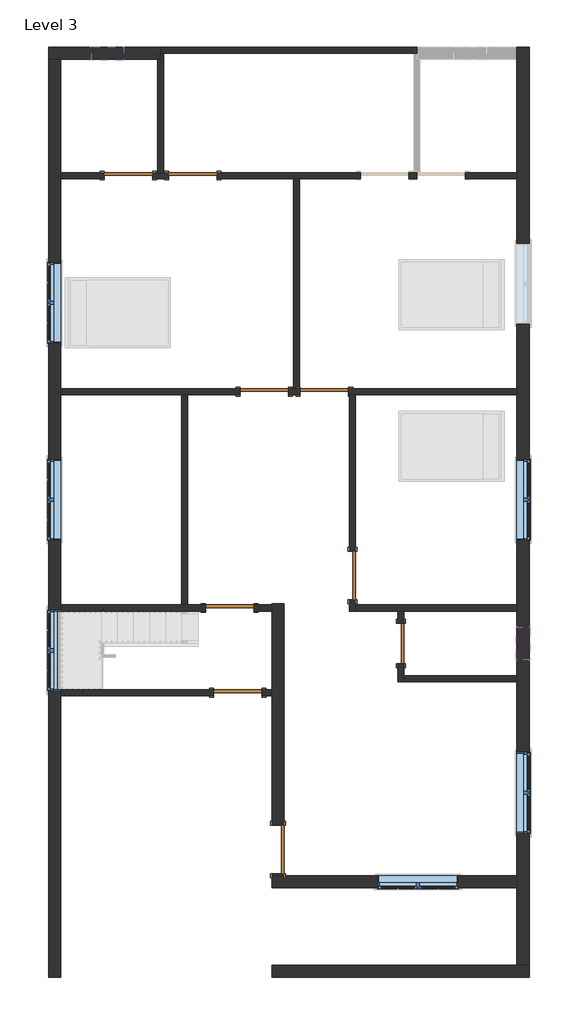
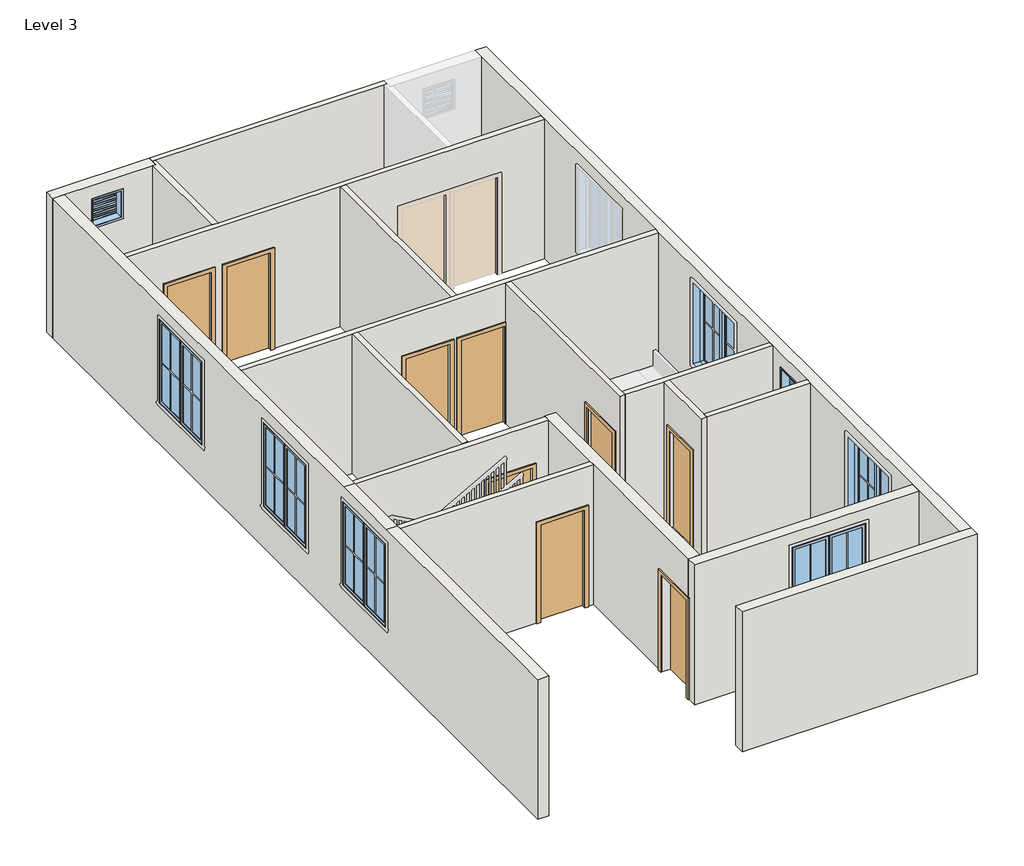
# One storey, part 1 of 3: 18 walls, 9 doors, 8 windows.
"""IFC4 building model written with IfcOpenShell, lengths in millimetres."""

from ifc_helpers import new_model, si_unit, frame, origin, place, context, project, spatial, polyline, outline, extrude, faceted_brep, transform, mapped, element, save
from components import door_78caadf7, single_flush_door_3_e5f9f3c4, single_flush_door_3_305aa2a5, single_flush_door_3_0ca8825f, window_casement_double_win_5_f93960c7, window_f2d8fef0

model = new_model("IFC4")

# Units and contexts
model_context = context("Model", 3, world=origin())
ifc_project = project(units=[si_unit("LENGTHUNIT", "METRE", prefix="MILLI")], contexts=[model_context])

# Site, building, storey
site = spatial("IfcSite", under=ifc_project)
building = spatial("IfcBuilding", under=site)
storey = spatial("IfcBuildingStorey", under=building, Name="Level 3", Elevation=3200.4)

# Doors
placement = place(None, origin())
door_shape = door_78caadf7(model_context)
element("IfcDoor", 1, ObjectType="Single-Flush : DOOR 2'6\"", at=placement, inside=storey, context=model_context, shape_type="MappedRepresentation", body=[
    mapped(door_shape, transform((860.2379845, -2779.6065691, 3200.4), x_axis=(0.0, 1.0, 0.0), y_axis=(-1.0, 0.0, 0.0), z_axis=(0.0, 0.0, 1.0))),
])
single_flush_door_3_shape = single_flush_door_3_e5f9f3c4(model_context)
element("IfcDoor", 2, ObjectType="Single-Flush : DOOR 3'", at=placement, inside=storey, context=model_context, shape_type="MappedRepresentation", body=[
    mapped(single_flush_door_3_shape, transform((-54.1620155, -1503.2565691, 3200.4), x_axis=(0.0, -1.0, 0.0), y_axis=(1.0, 0.0, 0.0), z_axis=(0.0, 0.0, 1.0))),
])
element("IfcDoor", 3, ObjectType="Single-Flush : DOOR 3'", at=placement, inside=storey, context=model_context, shape_type="MappedRepresentation", body=[
    mapped(single_flush_door_3_shape, transform((-1717.8620155, 1963.8434309, 3200.4), x_axis=(1.0, 0.0, 0.0), y_axis=(0.0, 1.0, 0.0), z_axis=(0.0, 0.0, 1.0))),
])
element("IfcDoor", 4, ObjectType="Single-Flush : DOOR 3'", at=placement, inside=storey, context=model_context, shape_type="MappedRepresentation", body=[
    mapped(single_flush_door_3_shape, transform((-2371.9120155, -2112.8565691, 3200.4), x_axis=(1.0, 0.0, 0.0), y_axis=(0.0, 1.0, 0.0), z_axis=(0.0, 0.0, 1.0))),
])
element("IfcDoor", 5, ObjectType="Single-Flush : DOOR 3'", at=placement, inside=storey, context=model_context, shape_type="MappedRepresentation", body=[
    mapped(single_flush_door_3_shape, transform((-2219.5120155, -3713.0565691, 3200.4), x_axis=(1.0, 0.0, 0.0), y_axis=(0.0, 1.0, 0.0), z_axis=(0.0, 0.0, 1.0))),
])
element("IfcDoor", 6, ObjectType="Single-Flush : DOOR 3'", at=placement, inside=storey, context=model_context, shape_type="MappedRepresentation", body=[
    mapped(single_flush_door_3_shape, transform((-4283.2620155, 6040.5434309, 3200.4), x_axis=(1.0, 0.0, 0.0), y_axis=(0.0, 1.0, 0.0), z_axis=(0.0, 0.0, 1.0))),
])
single_flush_door_3_2_shape = single_flush_door_3_305aa2a5(model_context)
element("IfcDoor", 7, ObjectType="Single-Flush : DOOR 3'", at=placement, inside=storey, context=model_context, shape_type="MappedRepresentation", body=[
    mapped(single_flush_door_3_2_shape, transform((-581.2120155, 1963.8434309, 3200.4), x_axis=(-1.0, 0.0, 0.0), y_axis=(0.0, -1.0, 0.0), z_axis=(0.0, 0.0, 1.0))),
])
element("IfcDoor", 8, ObjectType="Single-Flush : DOOR 3'", at=placement, inside=storey, context=model_context, shape_type="MappedRepresentation", body=[
    mapped(single_flush_door_3_2_shape, transform((-3064.0620155, 6040.5434309, 3200.4), x_axis=(-1.0, 0.0, 0.0), y_axis=(0.0, -1.0, 0.0), z_axis=(0.0, 0.0, 1.0))),
])
single_flush_door_3_3_shape = single_flush_door_3_0ca8825f(model_context)
element("IfcDoor", 9, ObjectType="Single-Flush : DOOR 3'", at=placement, inside=storey, context=model_context, shape_type="MappedRepresentation", body=[
    mapped(single_flush_door_3_3_shape, transform((-1457.5120155, -6665.8065691, 3200.4), x_axis=(0.0, -1.0, 0.0), y_axis=(1.0, 0.0, 0.0), z_axis=(0.0, 0.0, 1.0))),
])

# Walls
element("IfcWall", 10, ObjectType="WALL 4.5\"", at=placement, inside=storey, context=model_context, shape_type="Brep", body=[
    faceted_brep([(-3673.6620155, 8345.5934309, 3200.4), (-3616.5120155, 8345.5934309, 3200.4), (1107.8879845, 8345.5934309, 3200.4), (1165.0379845, 8345.5934309, 3200.4), (1165.0379845, 8345.5934309, 6248.4), (1107.8879845, 8345.5934309, 6248.4), (-3616.5120155, 8345.5934309, 6248.4), (-3673.6620155, 8345.5934309, 6248.4), (-3673.6620155, 8459.8934309, 3200.4), (-3673.6620155, 8459.8934309, 6248.4), (1165.0379845, 8459.8934309, 6248.4), (1165.0379845, 8459.8934309, 3200.4)], [[[0, 1, 2, 3, 4, 5, 6, 7]], [[8, 9, 10, 11]], [[3, 2, 1, 0, 8, 11]], [[4, 3, 11, 10]], [[0, 7, 9, 8]], [[7, 6, 5, 4, 10, 9]]]),
])
element("IfcWall", 11, ObjectType="WALL 4.5\"", at=placement, inside=storey, context=model_context, shape_type="SweptSolid", body=[
    extrude(outline(polyline([(-3730.8120155, 6097.6934309), (-3730.8120155, 8231.2934309), (-3673.6620155, 8231.2934309), (-3673.6620155, 8345.5934309), (-3616.5120155, 8345.5934309), (-3616.5120155, 6097.6934309), (-3730.8120155, 6097.6934309)])), frame((0.0, 0.0, 3200.4), z_axis=(0.0, 0.0, 1.0), x_axis=(1.0, 0.0, 0.0)), (0.0, 0.0, 1.0), 3048.0),
])
element("IfcWall", 12, ObjectType="WALL 4.5\"", at=placement, inside=storey, context=model_context, shape_type="Brep", body=[
    faceted_brep([(1165.0379845, 6097.6934309, 5334.0), (1165.0379845, 6097.6934309, 3200.4), (1107.8879845, 6097.6934309, 3200.4), (1012.6379845, 6097.6934309, 3200.4), (1012.6379845, 6097.6934309, 5334.0), (98.2379845, 6097.6934309, 5334.0), (98.2379845, 6097.6934309, 3200.4), (-2606.8620155, 6097.6934309, 3200.4), (-2606.8620155, 6097.6934309, 5334.0), (-3521.2620155, 6097.6934309, 5334.0), (-3521.2620155, 6097.6934309, 3200.4), (-3616.5120155, 6097.6934309, 3200.4), (-3730.8120155, 6097.6934309, 3200.4), (-3826.0620155, 6097.6934309, 3200.4), (-3826.0620155, 6097.6934309, 5334.0), (-4740.4620155, 6097.6934309, 5334.0), (-4740.4620155, 6097.6934309, 3200.4), (-5559.6120155, 6097.6934309, 3200.4), (-5559.6120155, 6097.6934309, 6248.4), (-3730.8120155, 6097.6934309, 6248.4), (-3616.5120155, 6097.6934309, 6248.4), (1107.8879845, 6097.6934309, 6248.4), (1222.1879845, 6097.6934309, 6248.4), (3050.9879845, 6097.6934309, 6248.4), (3050.9879845, 6097.6934309, 3200.4), (2079.4379845, 6097.6934309, 3200.4), (2079.4379845, 6097.6934309, 5334.0), (1012.6379845, 5983.3934309, 3200.4), (1165.0379845, 5983.3934309, 3200.4), (1165.0379845, 5983.3934309, 5334.0), (2079.4379845, 5983.3934309, 5334.0), (2079.4379845, 5983.3934309, 3200.4), (3050.9879845, 5983.3934309, 3200.4), (3050.9879845, 5983.3934309, 6248.4), (-1051.1120155, 5983.3934309, 6248.4), (-1165.4120155, 5983.3934309, 6248.4), (-5559.6120155, 5983.3934309, 6248.4), (-5559.6120155, 5983.3934309, 3200.4), (-4740.4620155, 5983.3934309, 3200.4), (-4740.4620155, 5983.3934309, 5334.0), (-3826.0620155, 5983.3934309, 5334.0), (-3826.0620155, 5983.3934309, 3200.4), (-3521.2620155, 5983.3934309, 3200.4), (-3521.2620155, 5983.3934309, 5334.0), (-2606.8620155, 5983.3934309, 5334.0), (-2606.8620155, 5983.3934309, 3200.4), (-1165.4120155, 5983.3934309, 3200.4), (-1051.1120155, 5983.3934309, 3200.4), (98.2379845, 5983.3934309, 3200.4), (98.2379845, 5983.3934309, 5334.0), (1012.6379845, 5983.3934309, 5334.0)], [[[0, 1, 2, 3, 4, 5, 6, 7, 8, 9, 10, 11, 12, 13, 14, 15, 16, 17, 18, 19, 20, 21, 22, 23, 24, 25, 26]], [[27, 28, 29, 30, 31, 32, 33, 34, 35, 36, 37, 38, 39, 40, 41, 42, 43, 44, 45, 46, 47, 48, 49, 50]], [[38, 37, 17, 16]], [[13, 12, 11, 10, 42, 41]], [[48, 47, 46, 45, 7, 6]], [[25, 24, 32, 31]], [[3, 2, 1, 28, 27]], [[18, 17, 37, 36]], [[24, 23, 33, 32]], [[14, 13, 41, 40]], [[15, 14, 40, 39]], [[16, 15, 39, 38]], [[43, 42, 10, 9]], [[44, 43, 9, 8]], [[45, 44, 8, 7]], [[4, 3, 27, 50]], [[5, 4, 50, 49]], [[6, 5, 49, 48]], [[29, 28, 1, 0]], [[30, 29, 0, 26]], [[31, 30, 26, 25]], [[23, 22, 21, 20, 19, 18, 36, 35, 34, 33]]]),
])
element("IfcWall", 13, ObjectType="WALL 4.5\"", at=placement, inside=storey, context=model_context, shape_type="SweptSolid", body=[
    extrude(outline(polyline([(-1165.4120155, 2020.9934309), (-1165.4120155, 5983.3934309), (-1051.1120155, 5983.3934309), (-1051.1120155, 2020.9934309), (-1165.4120155, 2020.9934309)])), frame((0.0, 0.0, 3200.4), z_axis=(0.0, 0.0, 1.0), x_axis=(1.0, 0.0, 0.0)), (0.0, 0.0, 1.0), 3048.0),
])
element("IfcWall", 14, ObjectType="WALL 4.5\"", at=placement, inside=storey, context=model_context, shape_type="Brep", body=[
    faceted_brep([(-1260.6620155, 1906.6934309, 5334.0), (-1260.6620155, 1906.6934309, 3200.4), (-1038.4120155, 1906.6934309, 3200.4), (-1038.4120155, 1906.6934309, 5334.0), (-124.0120155, 1906.6934309, 5334.0), (-124.0120155, 1906.6934309, 3200.4), (-111.3120155, 1906.6934309, 3200.4), (2.9879845, 1906.6934309, 3200.4), (3050.9879845, 1906.6934309, 3200.4), (3050.9879845, 1906.6934309, 6248.4), (2.9879845, 1906.6934309, 6248.4), (-111.3120155, 1906.6934309, 6248.4), (-3159.3120155, 1906.6934309, 6248.4), (-3273.6120155, 1906.6934309, 6248.4), (-5559.6120155, 1906.6934309, 6248.4), (-5559.6120155, 1906.6934309, 3200.4), (-3273.6120155, 1906.6934309, 3200.4), (-3159.3120155, 1906.6934309, 3200.4), (-2175.0620155, 1906.6934309, 3200.4), (-2175.0620155, 1906.6934309, 5334.0), (-1038.4120155, 2020.9934309, 3200.4), (-1051.1120155, 2020.9934309, 3200.4), (-1165.4120155, 2020.9934309, 3200.4), (-1260.6620155, 2020.9934309, 3200.4), (-1260.6620155, 2020.9934309, 5334.0), (-2175.0620155, 2020.9934309, 5334.0), (-2175.0620155, 2020.9934309, 3200.4), (-5559.6120155, 2020.9934309, 3200.4), (-5559.6120155, 2020.9934309, 6248.4), (-1165.4120155, 2020.9934309, 6248.4), (-1051.1120155, 2020.9934309, 6248.4), (3050.9879845, 2020.9934309, 6248.4), (3050.9879845, 2020.9934309, 3200.4), (-124.0120155, 2020.9934309, 3200.4), (-124.0120155, 2020.9934309, 5334.0), (-1038.4120155, 2020.9934309, 5334.0)], [[[0, 1, 2, 3, 4, 5, 6, 7, 8, 9, 10, 11, 12, 13, 14, 15, 16, 17, 18, 19]], [[20, 21, 22, 23, 24, 25, 26, 27, 28, 29, 30, 31, 32, 33, 34, 35]], [[33, 32, 8, 7, 6, 5]], [[2, 1, 23, 22, 21, 20]], [[18, 17, 16, 15, 27, 26]], [[15, 14, 28, 27]], [[9, 8, 32, 31]], [[3, 2, 20, 35]], [[4, 3, 35, 34]], [[5, 4, 34, 33]], [[24, 23, 1, 0]], [[25, 24, 0, 19]], [[26, 25, 19, 18]], [[14, 13, 12, 11, 10, 9, 31, 30, 29, 28]]]),
])
element("IfcWall", 15, ObjectType="WALL 4.5\"", at=placement, inside=storey, context=model_context, shape_type="SweptSolid", body=[
    extrude(outline(polyline([(-3273.6120155, -2032.8465691), (-3273.6120155, 1906.6934309), (-3159.3120155, 1906.6934309), (-3159.3120155, -2032.8465691), (-3273.6120155, -2032.8465691)])), frame((0.0, 0.0, 3200.4), z_axis=(0.0, 0.0, 1.0), x_axis=(1.0, 0.0, 0.0)), (0.0, 0.0, 1.0), 3048.0),
])
element("IfcWall", 16, ObjectType="WALL 4.5\"", at=placement, inside=storey, context=model_context, shape_type="SweptSolid", body=[
    extrude(outline(polyline([(5334.0, -1914.7120155), (3200.4, -1914.7120155), (3200.4, -1571.8120155), (6248.4, -1571.8120155), (6248.4, -5559.6120155), (3200.4, -5559.6120155), (3200.4, -2829.1120155), (5334.0, -2829.1120155), (5334.0, -1914.7120155)])), frame((0.0, -2170.0065691, 0.0), z_axis=(0.0, 1.0, 0.0), x_axis=(0.0, 0.0, 1.0)), (0.0, 0.0, 1.0), 114.3),
])
element("IfcWall", 17, ObjectType="WALL 4.5\"", at=placement, inside=storey, context=model_context, shape_type="SweptSolid", body=[
    extrude(outline(polyline([(5334.0, -1762.3120155), (3200.4, -1762.3120155), (3200.4, -1571.8120155), (6248.4, -1571.8120155), (6248.4, -5559.6120155), (3200.4, -5559.6120155), (3200.4, -2676.7120155), (5334.0, -2676.7120155), (5334.0, -1762.3120155)])), frame((0.0, -3770.2065691, 0.0), z_axis=(0.0, 1.0, 0.0), x_axis=(0.0, 0.0, 1.0)), (0.0, 0.0, 1.0), 114.3),
])
element("IfcWall", 18, ObjectType="WALL 4.5\"", at=placement, inside=storey, context=model_context, shape_type="Brep", body=[
    faceted_brep([(-111.3120155, -1960.4565691, 5334.0), (-111.3120155, -1960.4565691, 3200.4), (-111.3120155, -2170.0065691, 3200.4), (-111.3120155, -2170.0065691, 6248.4), (-111.3120155, 1906.6934309, 6248.4), (-111.3120155, 1906.6934309, 3200.4), (-111.3120155, -1046.0565691, 3200.4), (-111.3120155, -1046.0565691, 5334.0), (2.9879845, -2170.0065691, 3200.4), (2.9879845, -2055.7065691, 3200.4), (2.9879845, -1960.4565691, 3200.4), (2.9879845, -1960.4565691, 5334.0), (2.9879845, -1046.0565691, 5334.0), (2.9879845, -1046.0565691, 3200.4), (2.9879845, 1906.6934309, 3200.4), (2.9879845, 1906.6934309, 6248.4), (2.9879845, -2055.7065691, 6248.4), (2.9879845, -2170.0065691, 6248.4)], [[[0, 1, 2, 3, 4, 5, 6, 7]], [[8, 9, 10, 11, 12, 13, 14, 15, 16, 17]], [[6, 5, 14, 13]], [[2, 1, 10, 9, 8]], [[5, 4, 15, 14]], [[3, 2, 8, 17]], [[11, 10, 1, 0]], [[12, 11, 0, 7]], [[13, 12, 7, 6]], [[4, 3, 17, 16, 15]]]),
])
element("IfcWall", 19, ObjectType="WALL 4.5\"", at=placement, inside=storey, context=model_context, shape_type="Brep", body=[
    faceted_brep([(2.9879845, -2170.0065691, 3200.4), (803.0879845, -2170.0065691, 3200.4), (917.3879845, -2170.0065691, 3200.4), (3050.9879845, -2170.0065691, 3200.4), (3050.9879845, -2170.0065691, 6248.4), (917.3879845, -2170.0065691, 6248.4), (803.0879845, -2170.0065691, 6248.4), (2.9879845, -2170.0065691, 6248.4), (2.9879845, -2055.7065691, 3200.4), (2.9879845, -2055.7065691, 6248.4), (3050.9879845, -2055.7065691, 6248.4), (3050.9879845, -2055.7065691, 3200.4)], [[[0, 1, 2, 3, 4, 5, 6, 7]], [[8, 9, 10, 11]], [[3, 2, 1, 0, 8, 11]], [[0, 7, 9, 8]], [[4, 3, 11, 10]], [[7, 6, 5, 4, 10, 9]]]),
])
element("IfcWall", 20, ObjectType="WALL 4.5\"", at=placement, inside=storey, context=model_context, shape_type="Brep", body=[
    faceted_brep([(803.0879845, -2170.0065691, 3200.4), (803.0879845, -2398.6065691, 3200.4), (803.0879845, -2398.6065691, 5334.0), (803.0879845, -3160.6065691, 5334.0), (803.0879845, -3160.6065691, 3200.4), (803.0879845, -3503.5065691, 3200.4), (803.0879845, -3503.5065691, 6248.4), (803.0879845, -2170.0065691, 6248.4), (917.3879845, -2398.6065691, 5334.0), (917.3879845, -2398.6065691, 3200.4), (917.3879845, -2170.0065691, 3200.4), (917.3879845, -2170.0065691, 6248.4), (917.3879845, -3389.2065691, 6248.4), (917.3879845, -3503.5065691, 6248.4), (917.3879845, -3503.5065691, 3200.4), (917.3879845, -3389.2065691, 3200.4), (917.3879845, -3160.6065691, 3200.4), (917.3879845, -3160.6065691, 5334.0)], [[[0, 1, 2, 3, 4, 5, 6, 7]], [[8, 9, 10, 11, 12, 13, 14, 15, 16, 17]], [[10, 9, 1, 0]], [[16, 15, 14, 5, 4]], [[0, 7, 11, 10]], [[6, 5, 14, 13]], [[2, 1, 9, 8]], [[3, 2, 8, 17]], [[4, 3, 17, 16]], [[7, 6, 13, 12, 11]]]),
])
element("IfcWall", 21, ObjectType="WALL 4.5\"", at=placement, inside=storey, context=model_context, shape_type="SweptSolid", body=[
    extrude(outline(polyline([(917.3879845, -3389.2065691), (3050.9879845, -3389.2065691), (3050.9879845, -3503.5065691), (917.3879845, -3503.5065691), (917.3879845, -3389.2065691)])), frame((0.0, 0.0, 3200.4), z_axis=(0.0, 0.0, 1.0), x_axis=(1.0, 0.0, 0.0)), (0.0, 0.0, 1.0), 3048.0),
])
element("IfcWall", 22, ObjectType="WALL 9\"", at=placement, inside=storey, context=model_context, shape_type="Brep", body=[
    faceted_brep([(-3673.6620155, 8459.8934309, 3200.4), (-5788.2120155, 8459.8934309, 3200.4), (-5788.2120155, 8459.8934309, 6248.4), (-3673.6620155, 8459.8934309, 6248.4), (-4978.5870155, 8459.8934309, 5943.6), (-4978.5870155, 8459.8934309, 5334.0), (-4368.9870155, 8459.8934309, 5334.0), (-4368.9870155, 8459.8934309, 5943.6), (-3673.6620155, 8231.2934309, 3200.4), (-3673.6620155, 8231.2934309, 6248.4), (-3730.8120155, 8231.2934309, 6248.4), (-5559.6120155, 8231.2934309, 6248.4), (-5788.2120155, 8231.2934309, 6248.4), (-5788.2120155, 8231.2934309, 3200.4), (-5559.6120155, 8231.2934309, 3200.4), (-3730.8120155, 8231.2934309, 3200.4), (-4978.5870155, 8231.2934309, 5943.6), (-4368.9870155, 8231.2934309, 5943.6), (-4368.9870155, 8231.2934309, 5334.0), (-4978.5870155, 8231.2934309, 5334.0), (-3673.6620155, 8345.5934309, 3200.4), (-3673.6620155, 8345.5934309, 6248.4)], [[[0, 1, 2, 3], [4, 5, 6, 7]], [[8, 9, 10, 11, 12, 13, 14, 15], [16, 17, 18, 19]], [[1, 0, 20, 8, 15, 14, 13]], [[0, 3, 21, 9, 8, 20]], [[2, 1, 13, 12]], [[5, 4, 16, 19]], [[6, 5, 19, 18]], [[7, 6, 18, 17]], [[4, 7, 17, 16]], [[3, 2, 12, 11, 10, 9, 21]]]),
])
element("IfcWall", 23, ObjectType="WALL 9\"", at=placement, inside=storey, context=model_context, shape_type="Brep", body=[
    faceted_brep([(-5788.2120155, 8231.2934309, 3200.4), (-5788.2120155, -9078.8065691, 3200.4), (-5788.2120155, -9078.8065691, 6248.4), (-5788.2120155, -3674.9565691, 6248.4), (-5788.2120155, -2150.9565691, 6248.4), (-5788.2120155, 8231.2934309, 6248.4), (-5788.2120155, 4402.2434309, 5943.6), (-5788.2120155, 2878.2434309, 5943.6), (-5788.2120155, 2878.2434309, 4114.8), (-5788.2120155, 4402.2434309, 4114.8), (-5788.2120155, -2150.9565691, 5943.6), (-5788.2120155, -3674.9565691, 5943.6), (-5788.2120155, -3674.9565691, 4114.8), (-5788.2120155, -2150.9565691, 4114.8), (-5788.2120155, 687.4934309, 5943.6), (-5788.2120155, -836.5065691, 5943.6), (-5788.2120155, -836.5065691, 4114.8), (-5788.2120155, 687.4934309, 4114.8), (-5559.6120155, 8231.2934309, 3200.4), (-5559.6120155, 8231.2934309, 6248.4), (-5559.6120155, 6097.6934309, 6248.4), (-5559.6120155, 5983.3934309, 6248.4), (-5559.6120155, 2020.9934309, 6248.4), (-5559.6120155, 1906.6934309, 6248.4), (-5559.6120155, -2055.7065691, 6248.4), (-5559.6120155, -2150.9565691, 6248.4), (-5559.6120155, -2170.0065691, 6248.4), (-5559.6120155, -3655.9065691, 6248.4), (-5559.6120155, -3674.9565691, 6248.4), (-5559.6120155, -3770.2065691, 6248.4), (-5559.6120155, -9078.8065691, 6248.4), (-5559.6120155, -9078.8065691, 3200.4), (-5559.6120155, -3770.2065691, 3200.4), (-5559.6120155, -3655.9065691, 3200.4), (-5559.6120155, -2170.0065691, 3200.4), (-5559.6120155, -2055.7065691, 3200.4), (-5559.6120155, 1906.6934309, 3200.4), (-5559.6120155, 2020.9934309, 3200.4), (-5559.6120155, 5983.3934309, 3200.4), (-5559.6120155, 6097.6934309, 3200.4), (-5559.6120155, 4402.2434309, 5943.6), (-5559.6120155, 4402.2434309, 4114.8), (-5559.6120155, 2878.2434309, 4114.8), (-5559.6120155, 2878.2434309, 5943.6), (-5559.6120155, -2150.9565691, 5943.6), (-5559.6120155, -2150.9565691, 4114.8), (-5559.6120155, -3674.9565691, 4114.8), (-5559.6120155, -3674.9565691, 5943.6), (-5559.6120155, 687.4934309, 5943.6), (-5559.6120155, 687.4934309, 4114.8), (-5559.6120155, -836.5065691, 4114.8), (-5559.6120155, -836.5065691, 5943.6)], [[[0, 1, 2, 3, 4, 5], [6, 7, 8, 9], [10, 11, 12, 13], [14, 15, 16, 17]], [[18, 19, 20, 21, 22, 23, 24, 25, 26, 27, 28, 29, 30, 31, 32, 33, 34, 35, 36, 37, 38, 39], [40, 41, 42, 43], [44, 45, 46, 47], [48, 49, 50, 51]], [[1, 0, 18, 39, 38, 37, 36, 35, 34, 33, 32, 31]], [[2, 1, 31, 30]], [[0, 5, 19, 18]], [[41, 40, 6, 9]], [[42, 41, 9, 8]], [[43, 42, 8, 7]], [[40, 43, 7, 6]], [[45, 44, 10, 13]], [[46, 45, 13, 12]], [[47, 46, 12, 11]], [[44, 47, 11, 10]], [[49, 48, 14, 17]], [[50, 49, 17, 16]], [[51, 50, 16, 15]], [[48, 51, 15, 14]], [[4, 3, 28, 27, 26, 25]], [[3, 2, 30, 29, 28]], [[5, 4, 25, 24, 23, 22, 21, 20, 19]]]),
])
element("IfcWall", 24, ObjectType="WALL 9\"", at=placement, inside=storey, context=model_context, shape_type="Brep", body=[
    faceted_brep([(-1571.8120155, -9078.8065691, 3200.4), (3279.5879845, -9078.8065691, 3200.4), (3279.5879845, -9078.8065691, 6248.4), (-1571.8120155, -9078.8065691, 6248.4), (-1571.8120155, -8850.2065691, 3200.4), (-1571.8120155, -8850.2065691, 6248.4), (3050.9879845, -8850.2065691, 6248.4), (3279.5879845, -8850.2065691, 6248.4), (3279.5879845, -8850.2065691, 3200.4), (3050.9879845, -8850.2065691, 3200.4)], [[[0, 1, 2, 3]], [[4, 5, 6, 7, 8, 9]], [[1, 0, 4, 9, 8]], [[0, 3, 5, 4]], [[2, 1, 8, 7]], [[3, 2, 7, 6, 5]]]),
])
element("IfcWall", 25, ObjectType="WALL 9\"", at=placement, inside=storey, context=model_context, shape_type="Brep", body=[
    faceted_brep([(3279.5879845, -8850.2065691, 3200.4), (3279.5879845, 8459.8934309, 3200.4), (3279.5879845, 8459.8934309, 6248.4), (3279.5879845, -8850.2065691, 6248.4), (3279.5879845, 3240.1934309, 5943.6), (3279.5879845, 4764.1934309, 5943.6), (3279.5879845, 4764.1934309, 4114.8), (3279.5879845, 3240.1934309, 4114.8), (3279.5879845, -836.5065691, 5943.6), (3279.5879845, 687.4934309, 5943.6), (3279.5879845, 687.4934309, 4114.8), (3279.5879845, -836.5065691, 4114.8), (3279.5879845, -6361.0065691, 5943.6), (3279.5879845, -4837.0065691, 5943.6), (3279.5879845, -4837.0065691, 4114.8), (3279.5879845, -6361.0065691, 4114.8), (3279.5879845, -2474.8065691, 5943.6), (3279.5879845, -2474.8065691, 5334.0), (3279.5879845, -3084.4065691, 5334.0), (3279.5879845, -3084.4065691, 5943.6), (3050.9879845, -8850.2065691, 3200.4), (3050.9879845, -8850.2065691, 6248.4), (3050.9879845, -7389.7065691, 6248.4), (3050.9879845, -7161.1065691, 6248.4), (3050.9879845, -3503.5065691, 6248.4), (3050.9879845, -3389.2065691, 6248.4), (3050.9879845, -2170.0065691, 6248.4), (3050.9879845, -2055.7065691, 6248.4), (3050.9879845, 1906.6934309, 6248.4), (3050.9879845, 2020.9934309, 6248.4), (3050.9879845, 5983.3934309, 6248.4), (3050.9879845, 6097.6934309, 6248.4), (3050.9879845, 8231.2934309, 6248.4), (3050.9879845, 8459.8934309, 6248.4), (3050.9879845, 8459.8934309, 3200.4), (3050.9879845, 8231.2934309, 3200.4), (3050.9879845, 6097.6934309, 3200.4), (3050.9879845, 5983.3934309, 3200.4), (3050.9879845, 2020.9934309, 3200.4), (3050.9879845, 1906.6934309, 3200.4), (3050.9879845, -2055.7065691, 3200.4), (3050.9879845, -2170.0065691, 3200.4), (3050.9879845, -3389.2065691, 3200.4), (3050.9879845, -3503.5065691, 3200.4), (3050.9879845, -7161.1065691, 3200.4), (3050.9879845, -7389.7065691, 3200.4), (3050.9879845, 3240.1934309, 5943.6), (3050.9879845, 3240.1934309, 4114.8), (3050.9879845, 4764.1934309, 4114.8), (3050.9879845, 4764.1934309, 5943.6), (3050.9879845, -836.5065691, 5943.6), (3050.9879845, -836.5065691, 4114.8), (3050.9879845, 687.4934309, 4114.8), (3050.9879845, 687.4934309, 5943.6), (3050.9879845, -6361.0065691, 5943.6), (3050.9879845, -6361.0065691, 4114.8), (3050.9879845, -4837.0065691, 4114.8), (3050.9879845, -4837.0065691, 5943.6), (3050.9879845, -2474.8065691, 5943.6), (3050.9879845, -3084.4065691, 5943.6), (3050.9879845, -3084.4065691, 5334.0), (3050.9879845, -2474.8065691, 5334.0)], [[[0, 1, 2, 3], [4, 5, 6, 7], [8, 9, 10, 11], [12, 13, 14, 15], [16, 17, 18, 19]], [[20, 21, 22, 23, 24, 25, 26, 27, 28, 29, 30, 31, 32, 33, 34, 35, 36, 37, 38, 39, 40, 41, 42, 43, 44, 45], [46, 47, 48, 49], [50, 51, 52, 53], [54, 55, 56, 57], [58, 59, 60, 61]], [[1, 0, 20, 45, 44, 43, 42, 41, 40, 39, 38, 37, 36, 35, 34]], [[0, 3, 21, 20]], [[2, 1, 34, 33]], [[47, 46, 4, 7]], [[48, 47, 7, 6]], [[49, 48, 6, 5]], [[46, 49, 5, 4]], [[51, 50, 8, 11]], [[52, 51, 11, 10]], [[53, 52, 10, 9]], [[50, 53, 9, 8]], [[55, 54, 12, 15]], [[56, 55, 15, 14]], [[57, 56, 14, 13]], [[54, 57, 13, 12]], [[17, 16, 58, 61]], [[18, 17, 61, 60]], [[19, 18, 60, 59]], [[16, 19, 59, 58]], [[3, 2, 33, 32, 31, 30, 29, 28, 27, 26, 25, 24, 23, 22, 21]]]),
])
element("IfcWall", 26, ObjectType="WALL 9\"", at=placement, inside=storey, context=model_context, shape_type="Brep", body=[
    faceted_brep([(3050.9879845, -7161.1065691, 3200.4), (-1343.2120155, -7161.1065691, 3200.4), (-1571.8120155, -7161.1065691, 3200.4), (-1571.8120155, -7161.1065691, 6248.4), (-1343.2120155, -7161.1065691, 6248.4), (3050.9879845, -7161.1065691, 6248.4), (422.0879845, -7161.1065691, 5943.6), (422.0879845, -7161.1065691, 4114.8), (1946.0879845, -7161.1065691, 4114.8), (1946.0879845, -7161.1065691, 5943.6), (3050.9879845, -7389.7065691, 3200.4), (3050.9879845, -7389.7065691, 6248.4), (-1571.8120155, -7389.7065691, 6248.4), (-1571.8120155, -7389.7065691, 3200.4), (422.0879845, -7389.7065691, 5943.6), (1946.0879845, -7389.7065691, 5943.6), (1946.0879845, -7389.7065691, 4114.8), (422.0879845, -7389.7065691, 4114.8)], [[[0, 1, 2, 3, 4, 5], [6, 7, 8, 9]], [[10, 11, 12, 13], [14, 15, 16, 17]], [[2, 1, 0, 10, 13]], [[0, 5, 11, 10]], [[3, 2, 13, 12]], [[7, 6, 14, 17]], [[8, 7, 17, 16]], [[9, 8, 16, 15]], [[6, 9, 15, 14]], [[5, 4, 3, 12, 11]]]),
])
element("IfcWall", 27, ObjectType="WALL 9\"", at=placement, inside=storey, context=model_context, shape_type="Brep", body=[
    faceted_brep([(-1343.2120155, -7161.1065691, 3200.4), (-1343.2120155, -7123.0065691, 3200.4), (-1343.2120155, -7123.0065691, 5334.0), (-1343.2120155, -6208.6065691, 5334.0), (-1343.2120155, -6208.6065691, 3200.4), (-1343.2120155, -2032.8465691, 3200.4), (-1343.2120155, -2032.8465691, 6248.4), (-1343.2120155, -7161.1065691, 6248.4), (-1571.8120155, -7123.0065691, 5334.0), (-1571.8120155, -7123.0065691, 3200.4), (-1571.8120155, -7161.1065691, 3200.4), (-1571.8120155, -7161.1065691, 6248.4), (-1571.8120155, -3770.2065691, 6248.4), (-1571.8120155, -3655.9065691, 6248.4), (-1571.8120155, -2170.0065691, 6248.4), (-1571.8120155, -2055.7065691, 6248.4), (-1571.8120155, -2032.8465691, 6248.4), (-1571.8120155, -2032.8465691, 3200.4), (-1571.8120155, -2055.7065691, 3200.4), (-1571.8120155, -2170.0065691, 3200.4), (-1571.8120155, -3655.9065691, 3200.4), (-1571.8120155, -3770.2065691, 3200.4), (-1571.8120155, -6208.6065691, 3200.4), (-1571.8120155, -6208.6065691, 5334.0)], [[[0, 1, 2, 3, 4, 5, 6, 7]], [[8, 9, 10, 11, 12, 13, 14, 15, 16, 17, 18, 19, 20, 21, 22, 23]], [[10, 9, 1, 0]], [[22, 21, 20, 19, 18, 17, 5, 4]], [[6, 5, 17, 16]], [[0, 7, 11, 10]], [[2, 1, 9, 8]], [[3, 2, 8, 23]], [[4, 3, 23, 22]], [[7, 6, 16, 15, 14, 13, 12, 11]]]),
])

# Windows
window_casement_double_win_5_shape = window_casement_double_win_5_f93960c7(model_context)
element("IfcWindow", 28, ObjectType="Window-Casement-Double : WIN 5'", at=placement, inside=storey, context=model_context, shape_type="MappedRepresentation", body=[
    mapped(window_casement_double_win_5_shape, transform((-5673.9120155, 3640.2434309, 3200.4), x_axis=(0.0, 1.0, 0.0), y_axis=(-1.0, 0.0, 0.0), z_axis=(0.0, 0.0, 1.0))),
])
element("IfcWindow", 29, ObjectType="Window-Casement-Double : WIN 5'", at=placement, inside=storey, context=model_context, shape_type="MappedRepresentation", body=[
    mapped(window_casement_double_win_5_shape, transform((3165.2879845, -74.5065691, 3200.4), x_axis=(0.0, -1.0, 0.0), y_axis=(1.0, 0.0, 0.0), z_axis=(0.0, 0.0, 1.0))),
])
element("IfcWindow", 30, ObjectType="Window-Casement-Double : WIN 5'", at=placement, inside=storey, context=model_context, shape_type="MappedRepresentation", body=[
    mapped(window_casement_double_win_5_shape, transform((3165.2879845, -5599.0065691, 3200.4), x_axis=(0.0, -1.0, 0.0), y_axis=(1.0, 0.0, 0.0), z_axis=(0.0, 0.0, 1.0))),
])
element("IfcWindow", 31, ObjectType="Window-Casement-Double : WIN 5'", at=placement, inside=storey, context=model_context, shape_type="MappedRepresentation", body=[
    mapped(window_casement_double_win_5_shape, transform((1184.0879845, -7275.4065691, 3200.4), x_axis=(-1.0, 0.0, 0.0), y_axis=(0.0, -1.0, 0.0), z_axis=(0.0, 0.0, 1.0))),
])
element("IfcWindow", 32, ObjectType="Window-Casement-Double : WIN 5'", at=placement, inside=storey, context=model_context, shape_type="MappedRepresentation", body=[
    mapped(window_casement_double_win_5_shape, transform((-5673.9120155, -2912.9565691, 3200.4), x_axis=(0.0, 1.0, 0.0), y_axis=(-1.0, 0.0, 0.0), z_axis=(0.0, 0.0, 1.0))),
])
element("IfcWindow", 33, ObjectType="Window-Casement-Double : WIN 5'", at=placement, inside=storey, context=model_context, shape_type="MappedRepresentation", body=[
    mapped(window_casement_double_win_5_shape, transform((-5673.9120155, -74.5065691, 3200.4), x_axis=(0.0, 1.0, 0.0), y_axis=(-1.0, 0.0, 0.0), z_axis=(0.0, 0.0, 1.0))),
])
window_shape = window_f2d8fef0(model_context)
element("IfcWindow", 34, ObjectType="Window-Louvers : 24\" x 24\"", at=placement, inside=storey, context=model_context, shape_type="MappedRepresentation", body=[
    mapped(window_shape, transform((-4673.7870155, 8351.9434309, 4419.6), x_axis=(1.0, 0.0, 0.0), y_axis=(0.0, 1.0, 0.0), z_axis=(0.0, 0.0, 1.0))),
])
element("IfcWindow", 35, ObjectType="Window-Louvers : 24\" x 24\"", at=placement, inside=storey, context=model_context, shape_type="MappedRepresentation", body=[
    mapped(window_shape, transform((3171.6379845, -2779.6065691, 4419.6), x_axis=(0.0, -1.0, 0.0), y_axis=(1.0, 0.0, 0.0), z_axis=(0.0, 0.0, 1.0))),
])

save(model, "model.ifc")

# Revit data of these elements
# Type "Single-Flush : DOOR 2'6\""
#   Type Mark = "10"
#   Construction Type Id = "MDOOR"
#   Assembly Code = "C1020"
#   Analytic Construction = "Metal"
#   Thickness = 0' - 2"
#   Heat Transfer Coefficient (U) = 0.651978 BTU/(h·ft²·°F)
#   Height = 7' - 0"
#   Trim Projection Ext = 0' - 1"
#   Trim Projection Int = 0' - 1"
#   Trim Width = 0' - 3"
#   Width = 2' - 6"
#   Define Thermal Properties by = 1
#   Door Material = Door - Panel
#   Frame Material = Door - Frame
#   Visual Light Transmittance = 0
#   Solar Heat Gain Coefficient = 0
#   Function = (empty or 0)
#   Wall Closure = (empty or 0)
# Type "Single-Flush : DOOR 3'"
#   Type Mark = "9"
#   Construction Type Id = "MDOOR"
#   Assembly Code = "C1020"
#   Analytic Construction = "Metal"
#   Thickness = 0' - 2"
#   Heat Transfer Coefficient (U) = 0.651978 BTU/(h·ft²·°F)
#   Height = 7' - 0"
#   Trim Projection Ext = 0' - 1"
#   Trim Projection Int = 0' - 1"
#   Trim Width = 0' - 3"
#   Width = 3' - 0"
#   Define Thermal Properties by = 1
#   Door Material = Door - Panel
#   Frame Material = Door - Frame
#   Visual Light Transmittance = 0
#   Solar Heat Gain Coefficient = 0
#   Function = (empty or 0)
#   Wall Closure = (empty or 0)
# Type "WALL 4.5\""
#   Assembly Code = "B2010"
#   Layers, outside or top first: 0' - 4 1/2" no material (function 1)
# Type "WALL 9\""
#   Assembly Code = "B2010"
#   Layers, outside or top first: 0' - 9" no material (function 1)
# Type "Window-Casement-Double : WIN 5'"
#   Type Mark = "18"
#   Fire Rating = "0.5h"
#   Assembly Code = "B2020100"
#   Analytic Construction = "Double glazing - domestic"
#   Frame Extension [instance default] = 0' - 0 1/4"
#   Window Inset [instance default] = 0' - 0"
#   Wall Thickness [instance default] = 0' - 6"
#   Interior Wall Closure [instance default] = 0' - 2 1/4"
#   Half Width = 2' - 6"
#   Visual Light Transmittance = 0.81
#   Thermal Resistance (R) = 1.8146 (h·ft²·°F)/BTU
#   Solar Heat Gain Coefficient = 0.76
#   Rough Width = 5' - 0 1/2"
#   Rough Height = 6' - 0 1/2"
#   Height = 6' - 0"
#   Heat Transfer Coefficient (U) = 0.5511 BTU/(h·ft²·°F)
#   Exterior Wall Closure [instance default] = 0' - 1 1/4"
#   Extension Jamb [instance default] = 0' - 2 1/4"
#   Default Sill Height = 3' - 0"
#   Width = 5' - 0"
#   Muntin Visibility = yes
#   Interior Trim Visibility [instance default] = yes
#   Exterior Trim Visibility [instance default] = yes
#   Extension Jamb Visibility [instance default] = yes
#   Interior Trim Material = Wood - Stained
#   Muntin Pattern = Muntin Pattern_2x2 : Muntin Pattern_2x2
#   Interior Trim = Trim-Window-Interior-Flat : Picture Frame
#   Interior Frame Material = Wood - Stained
#   Glass Panel Material = Glass
#   Exterior Trim Material = Clad - White
#   Exterior Trim = Trim-Window-Exterior-Flat : with Sill
#   Exterior Frame Material = Clad - White
#   Wall Closure = (empty or 0)
# Type "Window-Louvers : 24\" x 24\""
#   Type Mark = "19"
#   Construction Type Id = "GSP4R"
#   Assembly Code = "B20"
#   Analytic Construction = "1/8 in Pilkington single glazing"
#   Visual Light Transmittance = 0.9
#   Thermal Resistance (R) = 1.53941 (h·ft²·°F)/BTU
#   Solar Heat Gain Coefficient = 0.78
#   Max Height = 1' - 11.74264"
#   Height = 2' - 0"
#   Heat Transfer Coefficient (U) = 0.6496 BTU/(h·ft²·°F)
#   Blade Width [instance default] = 1' - 10 1/2"
#   Blade Vertical Thickness = 0' - 0.35355"
#   Blade Thickness = 0' - 0 1/4"
#   Blade Spacing = 0' - 1 1/2"
#   Blade Height = 0' - 1.85355"
#   Blade Depth = 0' - 3"
#   Blade Angle = 45.00°
#   Default Sill Height = 3' - 0"
#   Trim Projection_Exterior = 0' - 0 1/2"
#   Trim Projection_Interior = 0' - 0 1/2"
#   Trim Width_Exterior = 0' - 1 1/2"
#   Trim Width_Interior = 0' - 1 1/2"
#   Width = 2' - 0"
#   Max Blade Count = 12
#   Define Thermal Properties by = 1
#   Blade Count = 12
#   Frame Material = Birch
#   Louver Material = Birch
#   Trim Exterior Material = Birch
#   Trim Interior Material = Birch
#   Wall Closure = (empty or 0)
# Element 1 (IfcDoor, "Single-Flush : DOOR 2'6\"")
#   Phase Created = New Construction
#   Materials on its faces: "Door - Frame", "Door - Panel"
# Elements 2, 3, 4, 5, 6, 7, 8, 9 (IfcDoor, "Single-Flush : DOOR 3'")
#   Phase Created = New Construction
#   Materials on its faces: "Door - Frame", "Door - Panel"
# Elements 10, 17 (IfcWall, "WALL 4.5\"")
#   Top Offset = 0' - 0"
#   Base Offset = 0' - 0"
#   Unconnected Height = 10' - 0"
#   wall height = 10' - 0"
#   Phase Created = New Construction
#   Base Constraint = Level 3
#   Materials on its faces: "Default Wall", "Brick, Common"
# Elements 11, 12, 13, 14, 15, 16, 18, 19, 20, 21 (IfcWall, "WALL 4.5\"")
#   Top Offset = 0' - 0"
#   Base Offset = 0' - 0"
#   Unconnected Height = 10' - 0"
#   wall height = 10' - 0"
#   Phase Created = New Construction
#   Base Constraint = Level 3
#   Materials on its faces: "Default Wall"
# Elements 22, 23, 24, 25, 26, 27 (IfcWall, "WALL 9\"")
#   Top Offset = 0' - 0"
#   Base Offset = 0' - 0"
#   Unconnected Height = 10' - 0"
#   wall height = 10' - 0"
#   Phase Created = New Construction
#   Base Constraint = Level 3
#   Materials on its faces: "Default Wall", "Brick, Common"
# Element 28 (IfcWindow, "Window-Casement-Double : WIN 5'")
#   Mark = "11"
#   Window Inset = 0' - 0"
#   Interior Wall Closure = 0' - 2 1/4"
#   Frame Extension = 0' - 0 1/4"
#   Exterior Wall Closure = 0' - 1 1/4"
#   Interior Trim Visibility = yes
#   Exterior Trim Visibility = yes
#   Phase Created = New Construction
#   Materials on its faces: "Wood - Stained", "Glass", "Clad - White"
# Element 29 (IfcWindow, "Window-Casement-Double : WIN 5'")
#   Mark = "13"
#   Window Inset = 0' - 0"
#   Interior Wall Closure = 0' - 2 1/4"
#   Frame Extension = 0' - 0 1/4"
#   Exterior Wall Closure = 0' - 1 1/4"
#   Interior Trim Visibility = yes
#   Exterior Trim Visibility = yes
#   Phase Created = New Construction
#   Materials on its faces: "Wood - Stained", "Glass", "Clad - White"
# Element 30 (IfcWindow, "Window-Casement-Double : WIN 5'")
#   Mark = "14"
#   Window Inset = 0' - 0"
#   Interior Wall Closure = 0' - 2 1/4"
#   Frame Extension = 0' - 0 1/4"
#   Exterior Wall Closure = 0' - 1 1/4"
#   Interior Trim Visibility = yes
#   Exterior Trim Visibility = yes
#   Phase Created = New Construction
#   Materials on its faces: "Wood - Stained", "Glass", "Clad - White"
# Element 31 (IfcWindow, "Window-Casement-Double : WIN 5'")
#   Mark = "15"
#   Window Inset = 0' - 0"
#   Interior Wall Closure = 0' - 2 1/4"
#   Frame Extension = 0' - 0 1/4"
#   Exterior Wall Closure = 0' - 1 1/4"
#   Interior Trim Visibility = yes
#   Exterior Trim Visibility = yes
#   Phase Created = New Construction
#   Materials on its faces: "Wood - Stained", "Glass", "Clad - White"
# Element 32 (IfcWindow, "Window-Casement-Double : WIN 5'")
#   Mark = "16"
#   Window Inset = 0' - 0"
#   Interior Wall Closure = 0' - 2 1/4"
#   Frame Extension = 0' - 0 1/4"
#   Exterior Wall Closure = 0' - 1 1/4"
#   Interior Trim Visibility = yes
#   Exterior Trim Visibility = yes
#   Phase Created = New Construction
#   Materials on its faces: "Wood - Stained", "Glass", "Clad - White"
# Element 33 (IfcWindow, "Window-Casement-Double : WIN 5'")
#   Mark = "17"
#   Window Inset = 0' - 0"
#   Interior Wall Closure = 0' - 2 1/4"
#   Frame Extension = 0' - 0 1/4"
#   Exterior Wall Closure = 0' - 1 1/4"
#   Interior Trim Visibility = yes
#   Exterior Trim Visibility = yes
#   Phase Created = New Construction
#   Materials on its faces: "Wood - Stained", "Glass", "Clad - White"
# Element 34 (IfcWindow, "Window-Louvers : 24\" x 24\"")
#   Mark = "18"
#   Blade Width = 1' - 10 1/2"
#   Phase Created = New Construction
#   Materials on its faces: "Birch"
# Element 35 (IfcWindow, "Window-Louvers : 24\" x 24\"")
#   Mark = "20"
#   Blade Width = 1' - 10 1/2"
#   Phase Created = New Construction
#   Materials on its faces: "Birch"
# Materials
#   "Door - Panel": class "Wood", colour RGB 210 159 95, transparency 0, Cost = 0
#   "Door - Frame": colour RGB 118 70 51, transparency 0, Cost = 0
#   "Wood - Stained": class "Wood", colour RGB 224 178 126, transparency 0, Cost = 0
#   "Glass": class "Glass", colour RGB 0 128 192, transparency 0.75, Description = "Soda Lime Glass", Cost = 0
#   "Clad - White": class "Wood", colour RGB 242 242 238, transparency 0, Cost = 0
#   "Birch": class "Wood", colour RGB 224 178 126, transparency 0, Description = "Betula Alleghaniensis", Cost = 0
#   "Default Wall": colour RGB 128 128 128, transparency 0, Cost = 0
#   "Brick, Common": class "Masonry", colour RGB 170 98 104, transparency 0, Description = "Common brick", Cost = 0
